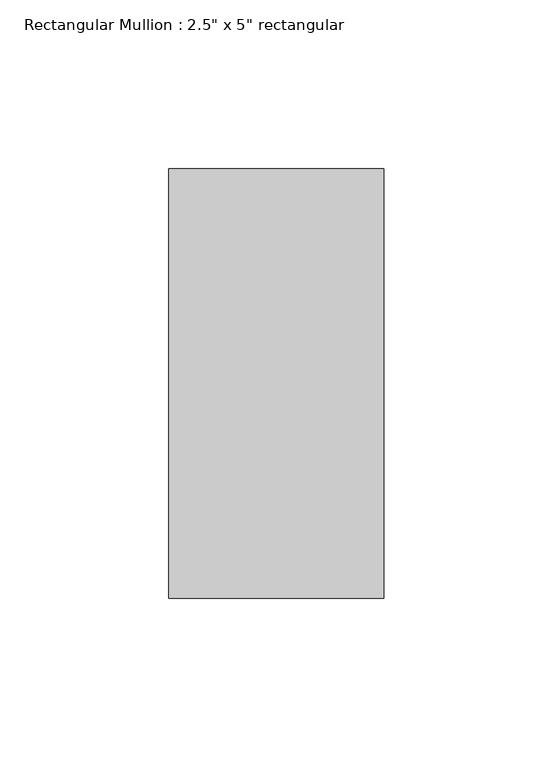
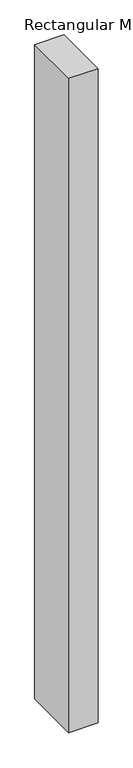
"""IFC4 building model written with IfcOpenShell, lengths in millimetres: member geometry."""

from ifc_helpers import new_model, si_unit, frame, origin, place, context, project, spatial, polyline, outline, extrude, source, transform, mapped, element, save


def member_8bf3bd84(model_context):
    return source(origin(), model_context, "Body", "SweptSolid", [
        extrude(outline(polyline([(31.75, 63.5), (31.75, -63.5), (-31.75, -63.5), (-31.75, 63.5), (31.75, 63.5)])), frame((0.0, 0.0, -1498.695751), z_axis=(0.0, 0.0, 1.0), x_axis=(1.0, 0.0, 0.0)), (0.0, 0.0, 1.0), 1498.695751),
    ])


if __name__ == "__main__":
    model = new_model("IFC4")
    model_context = context("Model", 3, world=origin())
    ifc_project = project(units=[si_unit("LENGTHUNIT", "METRE", prefix="MILLI")], contexts=[model_context])
    site = spatial("IfcSite", under=ifc_project)
    building = spatial("IfcBuilding", under=site)
    placement = place(None, origin())
    member_shape = member_8bf3bd84(model_context)
    element("IfcMember", 1, ObjectType="Rectangular Mullion : 2.5\" x 5\" rectangular", at=placement, inside=building, context=model_context, shape_type="MappedRepresentation", body=[
        mapped(member_shape, transform((0.0, 0.0, 0.0), x_axis=(1.0, 0.0, 0.0), y_axis=(0.0, 1.0, 0.0), z_axis=(0.0, 0.0, 1.0))),
    ])
    save(model, "model.ifc")

# Revit data of these elements
# Type "Rectangular Mullion : 2.5\" x 5\" rectangular"
#   built-in parameter 1007304 = 0.416667 (stored number, unit not read)
#   built-in parameter 1007301 = 0.104167 (stored number, unit not read)
#   built-in parameter 1007300 = 0.104167 (stored number, unit not read)
# Element 1 (IfcMember, "Rectangular Mullion : 2.5\" x 5\" rectangular")
#   Materials on its faces: "Aluminum"
# Materials
#   "Aluminum": class "Metal", colour RGB 247 247 247, transparency 0, Description = "Aluminum 6061", Cost = 0
